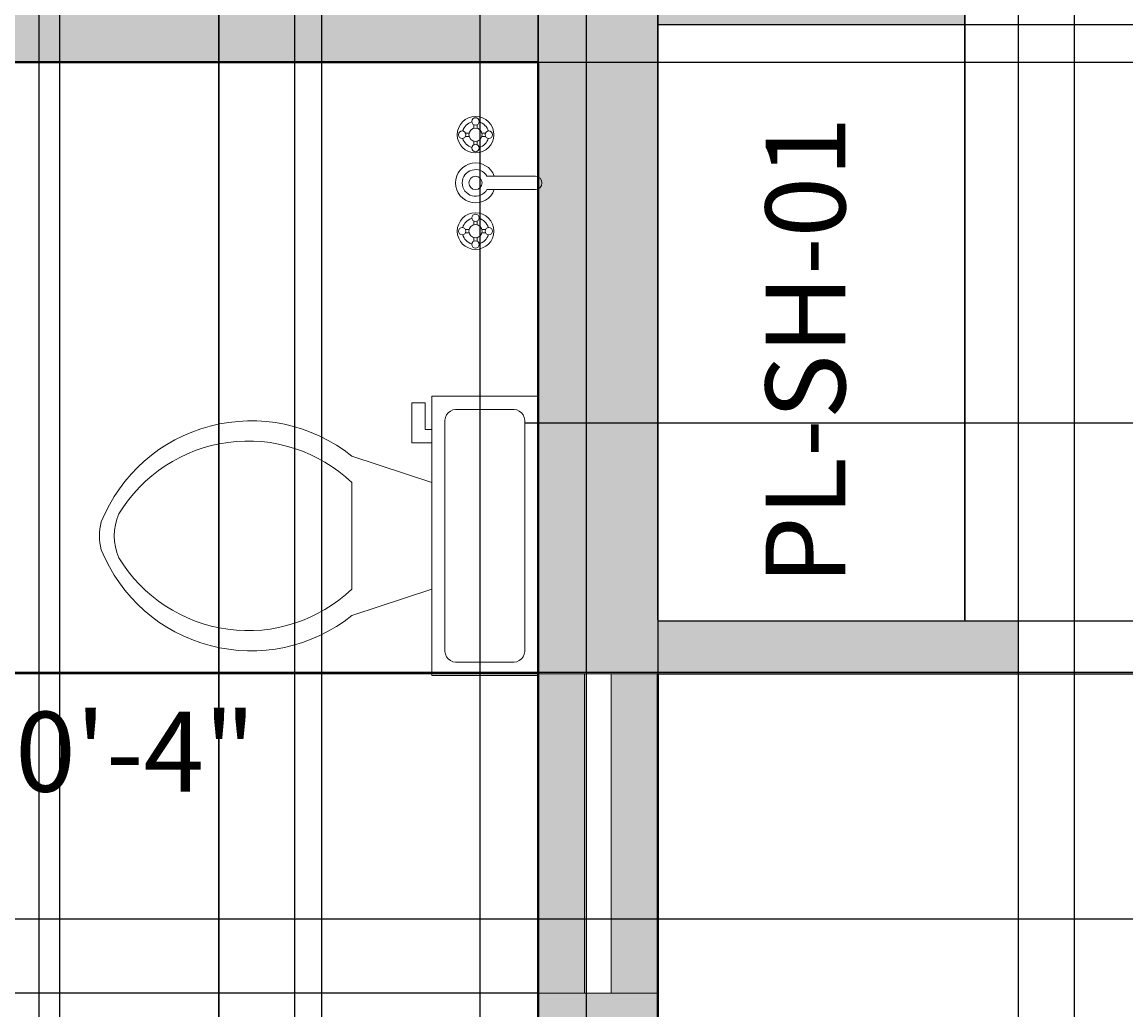
# Model space of a CAD drawing. Units: inches. Extents: x 818 to 1898, y 976 to 2364.
# Tile 46 of 96: x 1667 to 1750, y 1520 to 1594. Entities that reach past the tile are written whole.
import ezdxf

# ---------------------------------------------------------------- set-up
doc = ezdxf.new("R2010")
doc.units = ezdxf.units.IN
doc.header["$LTSCALE"] = 5
doc.header["$MEASUREMENT"] = 0
for name, color, linetype, lineweight in [('A-ANNO-DIMS', 2, 'Continuous', 18), ('A-ANNO-TEXT', 7, 'Continuous', 18), ('A-AREA-IDEN', 7, 'Continuous', 18), ('A-FLOR-FIXT', 9, 'Continuous', 18), ('A-FLOR-SHFT', 7, 'Continuous', 25), ('A-GLAZ', 4, 'Continuous', 18), ('A-WALL', 7, 'Continuous', 40)]:
    doc.layers.add(name, color=color, linetype=linetype, lineweight=lineweight)
doc.layers.add('A-GLAZ-PATT', color=141, linetype='Continuous', lineweight=9, true_color=0xadddf7)
doc.layers.add('A-WALL-PATT', color=251, linetype='Continuous', lineweight=13, true_color=0x636466)
doc.styles.get("Standard").update_dxf_attribs({"font": 'arial.ttf'})
doc.dimstyles.get("Standard").update_dxf_attribs({"dimtxt": 0.18, "dimasz": 0.18, "dimexe": 0.18, "dimexo": 0.0625, "dimgap": 0.09, "dimtad": 0, "dimtih": 1, "dimtoh": 1, "dimdec": 4, "dimzin": 0, "dimdsep": 46, "dimtxsty": 'Standard', "dimcen": 0.09, "dimadec": 0, "dimazin": 0, "dimtfac": 1, "dimtdec": 4, "dimtofl": 0, "dimtmove": 0, "dimatfit": 3, "dimfxl": 1, "dimtolj": 1, "dimtzin": 0, "dimarcsym": 0})

# ---------------------------------------------------------------- blocks, each defined once
blk = doc.blocks.new('Toilet - top')
for p, q in [((9.5, -6), (9.5, -2)), ((-8, -8.5), (-8, -8)), ((-7, -8), (-7, -9.5)), ((-4, -8), (-6, -14)), ((4, -8), (6, -14)), ((-10, -8.5), (-8, -8.5)), ((-10, -9.5), (-10, -8.5)), ((-7, -9.5), (-10, -9.5)), ((4, -14), (-4, -14))]:
    blk.add_line(p, q)
blk.add_lwpolyline([(10.5, -8), (10.5, 0), (-10.5, 0), (-10.5, -8)], close=True)
for points in [[(8.5, -1), (-8.5, -1)], [(-9.5, -2), (-9.5, -6)], [(-8.5, -7), (8.5, -7)]]:
    blk.add_lwpolyline(points)
for centre, radius, start, end in [((-8.625, -1.875), 0.884, 81.8699, 188.1301), ((8.625, -1.875), 0.884, 351.8699, 98.1301), ((-8.625, -6.125), 0.884, 171.8699, 278.1301), ((8.625, -6.125), 0.884, 261.8699, 8.1301), ((3.52, -21.58), 12.169, 141.46911, 247.97143), ((4.2, -21.817), 11.329, 136.36773, 238.94682), ((-3.519, -21.58), 12.169, 292.02843, 38.53071), ((-4.2, -21.817), 11.329, 301.05301, 43.63209), ((0, -27.876), 4, 245.73182, 294.26817), ((0, -29), 4, 254.86053, 285.13947)]:
    blk.add_arc(centre, radius, start, end)
blk = doc.blocks.new('Faucet - Bathroom top')
for p, q in [((-4.107, 0.125), (-4.375, 0.125)), ((-3.75, 0.4788), (-3.75, 0.75)), ((-3.5, 0.482), (-3.5, 0.75)), ((-3.1461, 0.125), (-2.875, 0.125)), ((3.143, 0.125), (2.875, 0.125)), ((3.5, 0.4788), (3.5, 0.75)), ((3.75, 0.482), (3.75, 0.75)), ((4.1039, 0.125), (4.375, 0.125)), ((-4.1039, -0.125), (-4.375, -0.125)), ((-3.75, -0.4821), (-3.75, -0.75)), ((-3.5, -0.4789), (-3.5, -0.75)), ((-3.143, -0.125), (-2.875, -0.125)), ((3.1461, -0.125), (2.875, -0.125)), ((3.5, -0.4821), (3.5, -0.75)), ((3.75, -0.4789), (3.75, -0.75)), ((4.107, -0.125), (4.375, -0.125)), ((-0.5, -0.8639), (-0.5, -4.5)), ((0.5, -4.5), (0.5, -0.8631))]:
    blk.add_line(p, q)
for centre, radius in [((-3.625, 0), 1.375), ((-3.625, 1), 0.2795), ((3.625, 0), 1.375), ((3.625, 1), 0.2795), ((-4.625, 0), 0.2795), ((-3.625, 0), 0.5), ((-2.625, 0), 0.2795), ((0, 0), 0.5), ((2.625, 0), 0.2795), ((3.625, 0), 0.5), ((4.625, 0), 0.2795), ((-3.625, -1), 0.2795), ((3.625, -1), 0.2795)]:
    blk.add_circle(centre, radius)
for centre, radius, start, end in [((-3.625, 0), 1, 105.2407, 164.2093), ((-3.625, 0), 1, 16.44125, 74.07887), ((0, 0), 1.5, 289.6514, 250.3603), ((0, 0), 1, 300.3431, 239.7554), ((3.625, 0), 1, 106.12, 164.0884), ((3.625, 0), 1, 16.23422, 73.90469), ((-3.625, 0), 1, 196.2342, 253.9047), ((-3.625, 0), 1, 286.12, 344.0884), ((3.625, 0), 1, 196.4413, 254.0789), ((3.625, 0), 1, 285.2407, 344.2093), ((0, -4.5), 0.5, 180, 0)]:
    blk.add_arc(centre, radius, start, end)
blk = doc.blocks.new('*D71')
at = {"layer": 'A-ANNO-DIMS', "color": 0, "lineweight": -2, "ltscale": 5, "transparency": 16777216}
for p, q in [((1714.788, 2053.078), (1897.916, 2053.078)), ((1897.736, 2052.898), (1897.736, 1699.76)), ((1897.736, 1346.258), (1897.736, 1699.396)), ((1714.788, 1346.078), (1897.916, 1346.078))]:
    blk.add_line(p, q, dxfattribs=at)
at = {"layer": 'A-ANNO-DIMS', "color": 0, "ltscale": 5, "transparency": 16777216}
for points in [[(1897.706, 2052.898), (1897.766, 2052.898), (1897.736, 2053.078)], [(1897.706, 1346.258), (1897.766, 1346.258), (1897.736, 1346.078)]]:
    blk.add_solid(points, dxfattribs=at)
at = {"layer": 'Defpoints', "color": 0, "ltscale": 5, "transparency": 16777216}
for p in [(1714.725, 2053.078), (1897.736, 2053.078), (1714.725, 1346.078)]:
    blk.add_point(p, dxfattribs=at)
at = {"layer": 'A-ANNO-DIMS', "color": 0, "ltscale": 5, "transparency": 16777216, "insert": (1897.736, 1699.578), "char_height": 0.18, "attachment_point": 5}
blk.add_mtext('\\A1;707', dxfattribs=at)
blk = doc.blocks.new('*D103')
at = {"layer": 'A-ANNO-DIMS', "color": 0, "lineweight": -2, "ltscale": 5, "transparency": 16777216}
for p, q in [((1626.575, 1071.118), (1626.575, 2363.873)), ((1626.755, 2363.693), (1657.699, 2363.693)), ((1689.291, 2363.693), (1658.348, 2363.693)), ((1689.471, 1071.118), (1689.471, 2363.873))]:
    blk.add_line(p, q, dxfattribs=at)
at = {"layer": 'A-ANNO-DIMS', "color": 0, "ltscale": 5, "transparency": 16777216}
for points in [[(1626.755, 2363.723), (1626.755, 2363.663), (1626.575, 2363.693)], [(1689.291, 2363.723), (1689.291, 2363.663), (1689.471, 2363.693)]]:
    blk.add_solid(points, dxfattribs=at)
at = {"layer": 'Defpoints', "color": 0, "ltscale": 5, "transparency": 16777216}
for p in [(1689.471, 2363.693), (1626.575, 1071.055), (1689.471, 1071.055)]:
    blk.add_point(p, dxfattribs=at)
at = {"layer": 'A-ANNO-DIMS', "color": 0, "ltscale": 5, "transparency": 16777216, "insert": (1658.023, 2363.693), "char_height": 0.18, "attachment_point": 5}
blk.add_mtext('\\A1;62.9', dxfattribs=at)
blk = doc.blocks.new('*D104')
at = {"layer": 'A-ANNO-DIMS', "color": 0, "lineweight": -2, "ltscale": 5, "transparency": 16777216}
for p, q in [((1689.471, 1071.118), (1689.471, 2363.873)), ((1689.651, 2363.693), (1717.401, 2363.693)), ((1745.903, 2363.693), (1718.154, 2363.693)), ((1746.083, 1071.118), (1746.083, 2363.873))]:
    blk.add_line(p, q, dxfattribs=at)
at = {"layer": 'A-ANNO-DIMS', "color": 0, "ltscale": 5, "transparency": 16777216}
for points in [[(1689.651, 2363.723), (1689.651, 2363.663), (1689.471, 2363.693)], [(1745.903, 2363.723), (1745.903, 2363.663), (1746.083, 2363.693)]]:
    blk.add_solid(points, dxfattribs=at)
at = {"layer": 'Defpoints', "color": 0, "ltscale": 5, "transparency": 16777216}
for p in [(1746.083, 2363.693), (1689.471, 1071.055), (1746.083, 1071.055)]:
    blk.add_point(p, dxfattribs=at)
at = {"layer": 'A-ANNO-DIMS', "color": 0, "ltscale": 5, "transparency": 16777216, "insert": (1717.777, 2363.693), "char_height": 0.18, "attachment_point": 5}
blk.add_mtext('\\A1;56.61', dxfattribs=at)
blk = doc.blocks.new('*D117')
at = {"layer": 'A-ANNO-DIMS', "color": 0, "lineweight": -2, "ltscale": 5, "transparency": 16777216}
for p, q in [((1766.29, 1545.183), (818.026, 1545.183)), ((818.206, 1545.003), (818.206, 1501.178)), ((818.206, 1456.989), (818.206, 1500.814)), ((1766.29, 1456.809), (818.026, 1456.809))]:
    blk.add_line(p, q, dxfattribs=at)
at = {"layer": 'A-ANNO-DIMS', "color": 0, "ltscale": 5, "transparency": 16777216}
for points in [[(818.176, 1545.003), (818.236, 1545.003), (818.206, 1545.183)], [(818.176, 1456.989), (818.236, 1456.989), (818.206, 1456.809)]]:
    blk.add_solid(points, dxfattribs=at)
at = {"layer": 'Defpoints', "color": 0, "ltscale": 5, "transparency": 16777216}
for p in [(818.206, 1545.183), (1766.352, 1545.183), (1766.352, 1456.809)]:
    blk.add_point(p, dxfattribs=at)
at = {"layer": 'A-ANNO-DIMS', "color": 0, "ltscale": 5, "transparency": 16777216, "insert": (818.206, 1500.996), "char_height": 0.18, "attachment_point": 5}
blk.add_mtext('\\A1;88.37', dxfattribs=at)
blk = doc.blocks.new('*D118')
at = {"layer": 'A-ANNO-DIMS', "color": 0, "lineweight": -2, "ltscale": 5, "transparency": 16777216}
for p, q in [((1766.29, 1627.505), (818.026, 1627.505)), ((818.206, 1627.325), (818.206, 1586.526)), ((818.206, 1545.363), (818.206, 1586.162)), ((1766.29, 1545.183), (818.026, 1545.183))]:
    blk.add_line(p, q, dxfattribs=at)
at = {"layer": 'A-ANNO-DIMS', "color": 0, "ltscale": 5, "transparency": 16777216}
for points in [[(818.176, 1627.325), (818.236, 1627.325), (818.206, 1627.505)], [(818.176, 1545.363), (818.236, 1545.363), (818.206, 1545.183)]]:
    blk.add_solid(points, dxfattribs=at)
at = {"layer": 'Defpoints', "color": 0, "ltscale": 5, "transparency": 16777216}
for p in [(818.206, 1627.505), (1766.352, 1627.505), (1766.352, 1545.183)]:
    blk.add_point(p, dxfattribs=at)
at = {"layer": 'A-ANNO-DIMS', "color": 0, "ltscale": 5, "transparency": 16777216, "insert": (818.206, 1586.344), "char_height": 0.18, "attachment_point": 5}
blk.add_mtext('\\A1;82.32', dxfattribs=at)
blk = doc.blocks.new('*D154')
at = {"layer": 'A-ANNO-DIMS', "color": 0, "lineweight": -2, "ltscale": 5, "transparency": 16777216}
for p, q in [((1701.369, 1290.141), (1701.369, 2363.873)), ((1701.549, 2363.693), (1705.22, 2363.693)), ((1709.189, 2363.693), (1705.518, 2363.693)), ((1709.369, 1298.141), (1709.369, 2363.873))]:
    blk.add_line(p, q, dxfattribs=at)
at = {"layer": 'A-ANNO-DIMS', "color": 0, "ltscale": 5, "transparency": 16777216}
for points in [[(1701.549, 2363.723), (1701.549, 2363.663), (1701.369, 2363.693)], [(1709.189, 2363.723), (1709.189, 2363.663), (1709.369, 2363.693)]]:
    blk.add_solid(points, dxfattribs=at)
at = {"layer": 'Defpoints', "color": 0, "ltscale": 5, "transparency": 16777216}
for p in [(1709.369, 2363.693), (1709.369, 1298.078), (1701.369, 1290.078)]:
    blk.add_point(p, dxfattribs=at)
at = {"layer": 'A-ANNO-DIMS', "color": 0, "ltscale": 5, "transparency": 16777216, "insert": (1705.369, 2363.693), "char_height": 0.18, "attachment_point": 5}
blk.add_mtext('\\A1;8', dxfattribs=at)
blk = doc.blocks.new('*D170')
at = {"layer": 'A-ANNO-DIMS', "color": 0, "lineweight": -2, "ltscale": 5, "transparency": 16777216}
for p, q in [((1430.788, 1600.078), (1897.916, 1600.078)), ((1897.736, 1599.898), (1897.736, 1550.76)), ((1897.736, 1501.258), (1897.736, 1550.396)), ((1430.788, 1501.078), (1897.916, 1501.078))]:
    blk.add_line(p, q, dxfattribs=at)
at = {"layer": 'A-ANNO-DIMS', "color": 0, "ltscale": 5, "transparency": 16777216}
for points in [[(1897.706, 1599.898), (1897.766, 1599.898), (1897.736, 1600.078)], [(1897.706, 1501.258), (1897.766, 1501.258), (1897.736, 1501.078)]]:
    blk.add_solid(points, dxfattribs=at)
at = {"layer": 'Defpoints', "color": 0, "ltscale": 5, "transparency": 16777216}
for p in [(1430.725, 1600.078), (1897.736, 1600.078), (1430.725, 1501.078)]:
    blk.add_point(p, dxfattribs=at)
at = {"layer": 'A-ANNO-DIMS', "color": 0, "ltscale": 5, "transparency": 16777216, "insert": (1897.736, 1550.578), "char_height": 0.18, "attachment_point": 5}
blk.add_mtext('\\A1;99', dxfattribs=at)
blk = doc.blocks.new('*D178')
at = {"layer": 'A-ANNO-DIMS', "color": 0, "lineweight": -2, "ltscale": 5, "transparency": 16777216}
for p, q in [((1669.725, 1600.016), (1669.725, 975.663)), ((1705.725, 1600.016), (1705.725, 975.663)), ((1669.905, 975.843), (1687.506, 975.843)), ((1705.545, 975.843), (1687.944, 975.843))]:
    blk.add_line(p, q, dxfattribs=at)
at = {"layer": 'A-ANNO-DIMS', "color": 0, "ltscale": 5, "transparency": 16777216}
for points in [[(1669.905, 975.873), (1669.905, 975.813), (1669.725, 975.843)], [(1705.545, 975.873), (1705.545, 975.813), (1705.725, 975.843)]]:
    blk.add_solid(points, dxfattribs=at)
at = {"layer": 'Defpoints', "color": 0, "ltscale": 5, "transparency": 16777216}
for p in [(1669.725, 1600.078), (1705.725, 1600.078), (1705.725, 975.843)]:
    blk.add_point(p, dxfattribs=at)
at = {"layer": 'A-ANNO-DIMS', "color": 0, "ltscale": 5, "transparency": 16777216, "insert": (1687.725, 975.843), "char_height": 0.18, "attachment_point": 5}
blk.add_mtext('\\A1;36', dxfattribs=at)
blk = doc.blocks.new('*D180')
at = {"layer": 'A-ANNO-DIMS', "color": 0, "lineweight": -2, "ltscale": 5, "transparency": 16777216}
for p, q in [((1599.725, 1639.516), (1599.725, 975.663)), ((1669.725, 1639.516), (1669.725, 975.663)), ((1599.905, 975.843), (1634.507, 975.843)), ((1669.545, 975.843), (1634.943, 975.843))]:
    blk.add_line(p, q, dxfattribs=at)
at = {"layer": 'A-ANNO-DIMS', "color": 0, "ltscale": 5, "transparency": 16777216}
for points in [[(1599.905, 975.873), (1599.905, 975.813), (1599.725, 975.843)], [(1669.545, 975.873), (1669.545, 975.813), (1669.725, 975.843)]]:
    blk.add_solid(points, dxfattribs=at)
at = {"layer": 'Defpoints', "color": 0, "ltscale": 5, "transparency": 16777216}
for p in [(1599.725, 1639.578), (1669.725, 1639.578), (1669.725, 975.843)]:
    blk.add_point(p, dxfattribs=at)
at = {"layer": 'A-ANNO-DIMS', "color": 0, "ltscale": 5, "transparency": 16777216, "insert": (1634.725, 975.843), "char_height": 0.18, "attachment_point": 5}
blk.add_mtext('\\A1;70', dxfattribs=at)
blk = doc.blocks.new('*D183')
at = {"layer": 'A-ANNO-DIMS', "color": 0, "lineweight": -2, "ltscale": 5, "transparency": 16777216}
for p, q in [((1714.725, 1545.016), (1714.725, 975.663)), ((1741.841, 1545.016), (1741.841, 975.663)), ((1714.905, 975.843), (1727.818, 975.843)), ((1741.661, 975.843), (1728.748, 975.843))]:
    blk.add_line(p, q, dxfattribs=at)
at = {"layer": 'A-ANNO-DIMS', "color": 0, "ltscale": 5, "transparency": 16777216}
for points in [[(1714.905, 975.873), (1714.905, 975.813), (1714.725, 975.843)], [(1741.661, 975.873), (1741.661, 975.813), (1741.841, 975.843)]]:
    blk.add_solid(points, dxfattribs=at)
at = {"layer": 'Defpoints', "color": 0, "ltscale": 5, "transparency": 16777216}
for p in [(1714.725, 1545.078), (1741.841, 1545.078), (1741.841, 975.843)]:
    blk.add_point(p, dxfattribs=at)
at = {"layer": 'A-ANNO-DIMS', "color": 0, "ltscale": 5, "transparency": 16777216, "insert": (1728.283, 975.843), "char_height": 0.18, "attachment_point": 5}
blk.add_mtext('\\A1;27.116', dxfattribs=at)
blk = doc.blocks.new('*D184')
at = {"layer": 'A-ANNO-DIMS', "color": 0, "lineweight": -2, "ltscale": 5, "transparency": 16777216}
for p, q in [((1737.903, 1593.918), (1897.916, 1593.918)), ((1897.736, 1593.738), (1897.736, 1571.68)), ((1897.736, 1549.258), (1897.736, 1571.316)), ((1737.903, 1549.078), (1897.916, 1549.078))]:
    blk.add_line(p, q, dxfattribs=at)
at = {"layer": 'A-ANNO-DIMS', "color": 0, "ltscale": 5, "transparency": 16777216}
for points in [[(1897.706, 1593.738), (1897.766, 1593.738), (1897.736, 1593.918)], [(1897.706, 1549.258), (1897.766, 1549.258), (1897.736, 1549.078)]]:
    blk.add_solid(points, dxfattribs=at)
at = {"layer": 'Defpoints', "color": 0, "ltscale": 5, "transparency": 16777216}
for p in [(1737.841, 1593.918), (1897.736, 1593.918), (1737.841, 1549.078)]:
    blk.add_point(p, dxfattribs=at)
at = {"layer": 'A-ANNO-DIMS', "color": 0, "ltscale": 5, "transparency": 16777216, "insert": (1897.736, 1571.498), "char_height": 0.18, "attachment_point": 5}
blk.add_mtext('\\A1;44.84', dxfattribs=at)
blk = doc.blocks.new('*D186')
at = {"layer": 'A-ANNO-DIMS', "color": 0, "lineweight": -2, "ltscale": 5, "transparency": 16777216}
for p, q in [((1714.725, 1549.141), (1714.725, 2363.873)), ((1714.905, 2363.693), (1725.818, 2363.693)), ((1737.661, 2363.693), (1726.748, 2363.693)), ((1737.841, 1549.141), (1737.841, 2363.873))]:
    blk.add_line(p, q, dxfattribs=at)
at = {"layer": 'A-ANNO-DIMS', "color": 0, "ltscale": 5, "transparency": 16777216}
for points in [[(1714.905, 2363.723), (1714.905, 2363.663), (1714.725, 2363.693)], [(1737.661, 2363.723), (1737.661, 2363.663), (1737.841, 2363.693)]]:
    blk.add_solid(points, dxfattribs=at)
at = {"layer": 'Defpoints', "color": 0, "ltscale": 5, "transparency": 16777216}
for p in [(1737.841, 2363.693), (1714.725, 1549.078), (1737.841, 1549.078)]:
    blk.add_point(p, dxfattribs=at)
at = {"layer": 'A-ANNO-DIMS', "color": 0, "ltscale": 5, "transparency": 16777216, "insert": (1726.283, 2363.693), "char_height": 0.18, "attachment_point": 5}
blk.add_mtext('\\A1;23.116', dxfattribs=at)
blk = doc.blocks.new('*D187')
at = {"layer": 'A-ANNO-DIMS', "color": 0, "lineweight": -2, "ltscale": 5, "transparency": 16777216}
for p, q in [((1705.663, 1545.078), (818.026, 1545.078)), ((818.206, 1544.898), (818.206, 1533.259)), ((818.206, 1521.258), (818.206, 1532.898)), ((1705.663, 1521.078), (818.026, 1521.078))]:
    blk.add_line(p, q, dxfattribs=at)
at = {"layer": 'A-ANNO-DIMS', "color": 0, "ltscale": 5, "transparency": 16777216}
for points in [[(818.176, 1544.898), (818.236, 1544.898), (818.206, 1545.078)], [(818.176, 1521.258), (818.236, 1521.258), (818.206, 1521.078)]]:
    blk.add_solid(points, dxfattribs=at)
at = {"layer": 'Defpoints', "color": 0, "ltscale": 5, "transparency": 16777216}
for p in [(818.206, 1545.078), (1705.725, 1545.078), (1705.725, 1521.078)]:
    blk.add_point(p, dxfattribs=at)
at = {"layer": 'A-ANNO-DIMS', "color": 0, "ltscale": 5, "transparency": 16777216, "insert": (818.206, 1533.078), "char_height": 0.18, "attachment_point": 5}
blk.add_mtext('\\A1;24', dxfattribs=at)
blk = doc.blocks.new('*D188')
at = {"layer": 'A-ANNO-DIMS', "color": 0, "lineweight": -2, "ltscale": 5, "transparency": 16777216}
for p, q in [((1714.788, 1545.078), (1897.916, 1545.078)), ((1897.736, 1544.898), (1897.736, 1445.76)), ((1897.736, 1346.258), (1897.736, 1445.396)), ((1714.788, 1346.078), (1897.916, 1346.078))]:
    blk.add_line(p, q, dxfattribs=at)
at = {"layer": 'A-ANNO-DIMS', "color": 0, "ltscale": 5, "transparency": 16777216}
for points in [[(1897.706, 1544.898), (1897.766, 1544.898), (1897.736, 1545.078)], [(1897.706, 1346.258), (1897.766, 1346.258), (1897.736, 1346.078)]]:
    blk.add_solid(points, dxfattribs=at)
at = {"layer": 'Defpoints', "color": 0, "ltscale": 5, "transparency": 16777216}
for p in [(1714.725, 1545.078), (1897.736, 1545.078), (1714.725, 1346.078)]:
    blk.add_point(p, dxfattribs=at)
at = {"layer": 'A-ANNO-DIMS', "color": 0, "ltscale": 5, "transparency": 16777216, "insert": (1897.736, 1445.578), "char_height": 0.18, "attachment_point": 5}
blk.add_mtext('\\A1;199', dxfattribs=at)
blk = doc.blocks.new('*D195')
at = {"layer": 'A-ANNO-DIMS', "color": 0, "lineweight": -2, "ltscale": 5, "transparency": 16777216}
for p, q in [((1681.725, 1379.141), (1681.725, 2363.873)), ((1681.905, 2363.693), (1693.505, 2363.693)), ((1705.545, 2363.693), (1693.945, 2363.693)), ((1705.725, 1355.141), (1705.725, 2363.873))]:
    blk.add_line(p, q, dxfattribs=at)
at = {"layer": 'A-ANNO-DIMS', "color": 0, "ltscale": 5, "transparency": 16777216}
for points in [[(1681.905, 2363.723), (1681.905, 2363.663), (1681.725, 2363.693)], [(1705.545, 2363.723), (1705.545, 2363.663), (1705.725, 2363.693)]]:
    blk.add_solid(points, dxfattribs=at)
at = {"layer": 'Defpoints', "color": 0, "ltscale": 5, "transparency": 16777216}
for p in [(1705.725, 2363.693), (1681.725, 1379.078), (1705.725, 1355.078)]:
    blk.add_point(p, dxfattribs=at)
at = {"layer": 'A-ANNO-DIMS', "color": 0, "ltscale": 5, "transparency": 16777216, "insert": (1693.725, 2363.693), "char_height": 0.18, "attachment_point": 5}
blk.add_mtext('\\A1;24', dxfattribs=at)
blk = doc.blocks.new('*D197')
at = {"layer": 'A-ANNO-DIMS', "color": 0, "lineweight": -2, "ltscale": 5, "transparency": 16777216}
for p, q in [((1457.788, 1526.671), (1897.916, 1526.671)), ((1897.736, 1526.491), (1897.736, 1468.076)), ((1897.736, 1409.298), (1897.736, 1467.713)), ((1457.788, 1409.118), (1897.916, 1409.118))]:
    blk.add_line(p, q, dxfattribs=at)
at = {"layer": 'A-ANNO-DIMS', "color": 0, "ltscale": 5, "transparency": 16777216}
for points in [[(1897.706, 1526.491), (1897.766, 1526.491), (1897.736, 1526.671)], [(1897.706, 1409.298), (1897.766, 1409.298), (1897.736, 1409.118)]]:
    blk.add_solid(points, dxfattribs=at)
at = {"layer": 'Defpoints', "color": 0, "ltscale": 5, "transparency": 16777216}
for p in [(1457.725, 1526.671), (1897.736, 1526.671), (1457.725, 1409.118)]:
    blk.add_point(p, dxfattribs=at)
at = {"layer": 'A-ANNO-DIMS', "color": 0, "ltscale": 5, "transparency": 16777216, "insert": (1897.736, 1467.894), "char_height": 0.18, "attachment_point": 5}
blk.add_mtext('\\A1;117.55', dxfattribs=at)
blk = doc.blocks.new('*D198')
at = {"layer": 'A-ANNO-DIMS', "color": 0, "lineweight": -2, "ltscale": 5, "transparency": 16777216}
for p, q in [((1741.841, 1545.016), (1741.841, 975.663)), ((1430.725, 1346.016), (1430.725, 975.663)), ((1430.905, 975.843), (1585.907, 975.843)), ((1741.661, 975.843), (1586.659, 975.843))]:
    blk.add_line(p, q, dxfattribs=at)
at = {"layer": 'A-ANNO-DIMS', "color": 0, "ltscale": 5, "transparency": 16777216}
for points in [[(1430.905, 975.873), (1430.905, 975.813), (1430.725, 975.843)], [(1741.661, 975.873), (1741.661, 975.813), (1741.841, 975.843)]]:
    blk.add_solid(points, dxfattribs=at)
at = {"layer": 'Defpoints', "color": 0, "ltscale": 5, "transparency": 16777216}
for p in [(1741.841, 1545.078), (1430.725, 1346.078), (1741.841, 975.843)]:
    blk.add_point(p, dxfattribs=at)
at = {"layer": 'A-ANNO-DIMS', "color": 0, "ltscale": 5, "transparency": 16777216, "insert": (1586.283, 975.843), "char_height": 0.18, "attachment_point": 5}
blk.add_mtext('\\A1;311.1', dxfattribs=at)
blk = doc.blocks.new('*D199')
at = {"layer": 'A-ANNO-DIMS', "color": 0, "lineweight": -2, "ltscale": 5, "transparency": 16777216}
for p, q in [((1559.788, 1687.078), (1897.916, 1687.078)), ((1897.736, 1686.898), (1897.736, 1513.154)), ((1897.736, 1339.045), (1897.736, 1512.79)), ((1660.377, 1338.865), (1897.916, 1338.865))]:
    blk.add_line(p, q, dxfattribs=at)
at = {"layer": 'A-ANNO-DIMS', "color": 0, "ltscale": 5, "transparency": 16777216}
for points in [[(1897.706, 1686.898), (1897.766, 1686.898), (1897.736, 1687.078)], [(1897.706, 1339.045), (1897.766, 1339.045), (1897.736, 1338.865)]]:
    blk.add_solid(points, dxfattribs=at)
at = {"layer": 'Defpoints', "color": 0, "ltscale": 5, "transparency": 16777216}
for p in [(1559.725, 1687.078), (1897.736, 1687.078), (1660.314, 1338.865)]:
    blk.add_point(p, dxfattribs=at)
at = {"layer": 'A-ANNO-DIMS', "color": 0, "ltscale": 5, "transparency": 16777216, "insert": (1897.736, 1512.972), "char_height": 0.18, "attachment_point": 5}
blk.add_mtext('\\A1;348.2', dxfattribs=at)
blk = doc.blocks.new('*D202')
at = {"layer": 'A-ANNO-DIMS', "color": 0, "lineweight": -2, "ltscale": 5, "transparency": 16777216}
for p, q in [((1705.788, 1591.078), (1897.916, 1591.078)), ((1897.736, 1590.898), (1897.736, 1577.702)), ((1897.736, 1564.146), (1897.736, 1577.342)), ((1704.788, 1563.966), (1897.916, 1563.966))]:
    blk.add_line(p, q, dxfattribs=at)
at = {"layer": 'A-ANNO-DIMS', "color": 0, "ltscale": 5, "transparency": 16777216}
for points in [[(1897.706, 1590.898), (1897.766, 1590.898), (1897.736, 1591.078)], [(1897.706, 1564.146), (1897.766, 1564.146), (1897.736, 1563.966)]]:
    blk.add_solid(points, dxfattribs=at)
at = {"layer": 'Defpoints', "color": 0, "ltscale": 5, "transparency": 16777216}
for p in [(1705.725, 1591.078), (1897.736, 1591.078), (1704.725, 1563.966)]:
    blk.add_point(p, dxfattribs=at)
at = {"layer": 'A-ANNO-DIMS', "color": 0, "ltscale": 5, "transparency": 16777216, "insert": (1897.736, 1577.522), "char_height": 0.18, "attachment_point": 5}
blk.add_mtext('\\A1;27.11', dxfattribs=at)
blk = doc.blocks.new('*D212')
at = {"layer": 'A-ANNO-DIMS', "color": 0, "lineweight": -2, "ltscale": 5, "transparency": 16777216}
for p, q in [((1681.725, 1900.016), (1681.725, 975.663)), ((1705.725, 1876.016), (1705.725, 975.663)), ((1681.905, 975.843), (1693.505, 975.843)), ((1705.545, 975.843), (1693.945, 975.843))]:
    blk.add_line(p, q, dxfattribs=at)
at = {"layer": 'A-ANNO-DIMS', "color": 0, "ltscale": 5, "transparency": 16777216}
for points in [[(1681.905, 975.873), (1681.905, 975.813), (1681.725, 975.843)], [(1705.545, 975.873), (1705.545, 975.813), (1705.725, 975.843)]]:
    blk.add_solid(points, dxfattribs=at)
at = {"layer": 'Defpoints', "color": 0, "ltscale": 5, "transparency": 16777216}
for p in [(1681.725, 1900.078), (1705.725, 1876.078), (1705.725, 975.843)]:
    blk.add_point(p, dxfattribs=at)
at = {"layer": 'A-ANNO-DIMS', "color": 0, "ltscale": 5, "transparency": 16777216, "insert": (1693.725, 975.843), "char_height": 0.18, "attachment_point": 5}
blk.add_mtext('\\A1;24', dxfattribs=at)
blk = doc.blocks.new('*D214')
at = {"layer": 'A-ANNO-DIMS', "color": 0, "lineweight": -2, "ltscale": 5, "transparency": 16777216}
for p, q in [((1511.725, 1687.016), (1511.725, 975.663)), ((1714.725, 1687.016), (1714.725, 975.663)), ((1511.905, 975.843), (1612.935, 975.843)), ((1714.545, 975.843), (1613.516, 975.843))]:
    blk.add_line(p, q, dxfattribs=at)
at = {"layer": 'A-ANNO-DIMS', "color": 0, "ltscale": 5, "transparency": 16777216}
for points in [[(1511.905, 975.873), (1511.905, 975.813), (1511.725, 975.843)], [(1714.545, 975.873), (1714.545, 975.813), (1714.725, 975.843)]]:
    blk.add_solid(points, dxfattribs=at)
at = {"layer": 'Defpoints', "color": 0, "ltscale": 5, "transparency": 16777216}
for p in [(1511.725, 1687.078), (1714.725, 1687.078), (1714.725, 975.843)]:
    blk.add_point(p, dxfattribs=at)
at = {"layer": 'A-ANNO-DIMS', "color": 0, "ltscale": 5, "transparency": 16777216, "insert": (1613.225, 975.843), "char_height": 0.18, "attachment_point": 5}
blk.add_mtext('\\A1;203', dxfattribs=at)
blk = doc.blocks.new('*D221')
at = {"layer": 'A-ANNO-DIMS', "color": 0, "lineweight": -2, "ltscale": 5, "transparency": 16777216}
for p, q in [((1668.184, 1696.016), (1668.184, 975.663)), ((1705.725, 1696.016), (1705.725, 975.663)), ((1668.364, 975.843), (1686.561, 975.843)), ((1705.545, 975.843), (1687.348, 975.843))]:
    blk.add_line(p, q, dxfattribs=at)
at = {"layer": 'A-ANNO-DIMS', "color": 0, "ltscale": 5, "transparency": 16777216}
for points in [[(1668.364, 975.873), (1668.364, 975.813), (1668.184, 975.843)], [(1705.545, 975.873), (1705.545, 975.813), (1705.725, 975.843)]]:
    blk.add_solid(points, dxfattribs=at)
at = {"layer": 'Defpoints', "color": 0, "ltscale": 5, "transparency": 16777216}
for p in [(1668.184, 1696.078), (1705.725, 1696.078), (1705.725, 975.843)]:
    blk.add_point(p, dxfattribs=at)
at = {"layer": 'A-ANNO-DIMS', "color": 0, "ltscale": 5, "transparency": 16777216, "insert": (1686.955, 975.843), "char_height": 0.18, "attachment_point": 5}
blk.add_mtext('\\A1;37.54', dxfattribs=at)
blk = doc.blocks.new('*D228')
at = {"layer": 'A-ANNO-DIMS', "color": 0, "lineweight": -2, "ltscale": 5, "transparency": 16777216}
for p, q in [((1687.394, 1802.016), (1687.394, 975.663)), ((1705.725, 1802.016), (1705.725, 975.663)), ((1687.574, 975.843), (1696.174, 975.843)), ((1705.545, 975.843), (1696.945, 975.843))]:
    blk.add_line(p, q, dxfattribs=at)
at = {"layer": 'A-ANNO-DIMS', "color": 0, "ltscale": 5, "transparency": 16777216}
for points in [[(1687.574, 975.873), (1687.574, 975.813), (1687.394, 975.843)], [(1705.545, 975.873), (1705.545, 975.813), (1705.725, 975.843)]]:
    blk.add_solid(points, dxfattribs=at)
at = {"layer": 'Defpoints', "color": 0, "ltscale": 5, "transparency": 16777216}
for p in [(1687.394, 1802.078), (1705.725, 1802.078), (1705.725, 975.843)]:
    blk.add_point(p, dxfattribs=at)
at = {"layer": 'A-ANNO-DIMS', "color": 0, "ltscale": 5, "transparency": 16777216, "insert": (1696.56, 975.843), "char_height": 0.18, "attachment_point": 5}
blk.add_mtext('\\A1;18.33', dxfattribs=at)
blk = doc.blocks.new('*D267')
at = {"layer": 'A-ANNO-DIMS', "color": 0, "lineweight": -2, "ltscale": 5, "transparency": 16777216}
for p, q in [((1714.725, 1687.016), (1714.725, 975.663)), ((1741.841, 1687.016), (1741.841, 975.663)), ((1714.905, 975.843), (1727.818, 975.843)), ((1741.661, 975.843), (1728.748, 975.843))]:
    blk.add_line(p, q, dxfattribs=at)
at = {"layer": 'A-ANNO-DIMS', "color": 0, "ltscale": 5, "transparency": 16777216}
for points in [[(1714.905, 975.873), (1714.905, 975.813), (1714.725, 975.843)], [(1741.661, 975.873), (1741.661, 975.813), (1741.841, 975.843)]]:
    blk.add_solid(points, dxfattribs=at)
at = {"layer": 'Defpoints', "color": 0, "ltscale": 5, "transparency": 16777216}
for p in [(1714.725, 1687.078), (1741.841, 1687.078), (1741.841, 975.843)]:
    blk.add_point(p, dxfattribs=at)
at = {"layer": 'A-ANNO-DIMS', "color": 0, "ltscale": 5, "transparency": 16777216, "insert": (1728.283, 975.843), "char_height": 0.18, "attachment_point": 5}
blk.add_mtext('\\A1;27.116', dxfattribs=at)

msp = doc.modelspace()

# ---------------------------------------------------------------- hatches: boundary and pattern name
at = {"layer": 'A-GLAZ-PATT', "ltscale": 5}
h = msp.add_hatch(color=256, dxfattribs=at)
h.dxf.hatch_style = 1
h.paths.add_polyline_path([(1283.8183, 1504.5782), (1206.7252, 1504.5782), (1206.7252, 1501.0782), (1283.8183, 1501.0782)])
h.paths.add_polyline_path([(1283.8183, 1510.0782), (1206.7252, 1510.0782), (1206.7252, 1506.5782), (1283.8183, 1506.5782)])
h.paths.add_polyline_path([(1490.9163, 1355.0782), (1439.7252, 1355.0782), (1439.7252, 1409.0522), (1436.2252, 1409.0522), (1436.2252, 1351.5782), (1490.9163, 1351.5782)])
h.paths.add_polyline_path([(1434.2252, 1409.0522), (1430.7251, 1409.0522), (1430.7251, 1346.0782), (1435.0799, 1346.0782), (1435.0731, 1346.1152), (1435.1501, 1346.0782), (1490.9163, 1346.0782), (1490.9163, 1349.5782), (1434.2252, 1349.5782)])
h.paths.add_polyline_path([(1714.7251, 1545.0782), (1711.2252, 1545.0782), (1711.2252, 1521.0782), (1714.7251, 1521.0782)])
h.paths.add_polyline_path([(1709.2252, 1545.0782), (1705.7251, 1545.0782), (1705.7251, 1521.0782), (1709.2252, 1521.0782)])
h.paths.add_polyline_path([(1714.7251, 1687.0782), (1711.2252, 1687.0782), (1711.2252, 1649.9029), (1714.7251, 1649.9029)])
h.paths.add_polyline_path([(1709.2252, 1687.0782), (1705.7251, 1687.0782), (1705.7251, 1649.9029), (1709.2252, 1649.9029)])
h.paths.add_polyline_path([(1709.2252, 1745.5584), (1705.7251, 1745.5584), (1705.7251, 1717.3178), (1709.2252, 1717.3178)])
h.paths.add_polyline_path([(1714.7251, 1745.5584), (1711.2252, 1745.5584), (1711.2252, 1717.3178), (1714.7251, 1717.3178)])
h.paths.add_polyline_path([(1714.7251, 2014.5114), (1711.2252, 2014.5114), (1711.2252, 1962.0338), (1714.7251, 1962.0338)])
h.paths.add_polyline_path([(1709.2252, 2014.5114), (1705.7251, 2014.5114), (1705.7251, 1962.0338), (1709.2252, 1962.0338)])
h.paths.add_polyline_path([(1538.5155, 2047.5782), (1485.1216, 2047.5782), (1485.1216, 2044.0782), (1538.5155, 2044.0782)])
h.paths.add_polyline_path([(1538.5155, 2053.0782), (1485.1216, 2053.0782), (1485.1216, 2049.5782), (1538.5155, 2049.5782)])
h.paths.add_polyline_path([(1388.0315, 2047.5782), (1330.305, 2047.5782), (1330.305, 2044.0782), (1388.0315, 2044.0782)])
h.paths.add_polyline_path([(1388.0315, 2053.0782), (1330.305, 2053.0782), (1330.305, 2049.5782), (1388.0315, 2049.5782)])
h.paths.add_polyline_path([(1262.2252, 2019.2871), (1258.7252, 2019.2871), (1258.7252, 1928.9218), (1262.2252, 1928.9218)])
h.paths.add_polyline_path([(1267.7252, 2019.2871), (1264.2252, 2019.2871), (1264.2252, 1928.9218), (1267.7252, 1928.9218)])
h.paths.add_polyline_path([(1262.2252, 1862.9652), (1258.7252, 1862.9652), (1258.7252, 1814.9652), (1262.2252, 1814.9652)])
h.paths.add_polyline_path([(1267.7252, 1862.9652), (1264.2252, 1862.9652), (1264.2252, 1814.9652), (1267.7252, 1814.9652)])
h.paths.add_polyline_path([(1262.2252, 1755.3321), (1258.7252, 1755.3321), (1258.7252, 1707.3321), (1262.2252, 1707.3321)])
h.paths.add_polyline_path([(1267.7252, 1755.3321), (1264.2252, 1755.3321), (1264.2252, 1707.3321), (1267.7252, 1707.3321)])
h.paths.add_polyline_path([(1251.9333, 1692.5782), (1206.7252, 1692.5782), (1206.7252, 1687.0782), (1251.9333, 1687.0782)])
h.paths.add_polyline_path([(1251.9333, 1700.0782), (1206.7252, 1700.0782), (1206.7252, 1694.5782), (1251.9333, 1694.5782)])
at = {"layer": 'A-WALL-PATT', "ltscale": 5}
h = msp.add_hatch(color=256, dxfattribs=at)
h.dxf.hatch_style = 1
h.paths.add_polyline_path([(1267.7252, 1928.9218), (1258.7252, 1928.9218), (1258.7252, 1913.6401), (1250.3029, 1913.6401), (1250.3029, 1878.3919), (1258.7252, 1878.3919), (1258.7252, 1862.9652), (1267.7252, 1862.9652)])
h.paths.add_polyline_path([(1267.7252, 1814.9652), (1258.7252, 1814.9652), (1258.7252, 1755.3321), (1267.7252, 1755.3321)])
h.paths.add_polyline_path([(1463.7252, 1696.0782), (1267.7252, 1696.0782), (1267.7252, 1707.3321), (1258.7252, 1707.3321), (1258.7252, 1700.0782), (1251.9333, 1700.0782), (1251.9333, 1687.0782), (1463.7252, 1687.0782)])
h.paths.add_polyline_path([(1714.7251, 1717.3178), (1705.7251, 1717.3178), (1705.7251, 1696.0782), (1599.7251, 1696.0782), (1599.7251, 1790.0782), (1705.7251, 1790.0782), (1705.7251, 1785.6125), (1714.7251, 1785.6125), (1714.7251, 1827.2125), (1705.7251, 1827.2125), (1705.7251, 1802.0782), (1599.7251, 1802.0782), (1599.7251, 1867.0782), (1705.7251, 1867.0782), (1705.7251, 1857.2125), (1714.7251, 1857.2125), (1714.7251, 1930.0316), (1741.8409, 1930.0316), (1741.8409, 1935.0316), (1714.7251, 1935.0316), (1714.7251, 1957.0338), (1741.8409, 1957.0338), (1741.8409, 1962.0338), (1714.7251, 1962.0338), (1705.7251, 1962.0338), (1705.7251, 1948.0782), (1599.7251, 1948.0782), (1599.7251, 1981.0782), (1590.7252, 1981.0782), (1590.7252, 1941.0782), (1620.7252, 1941.0782), (1705.7251, 1941.0782), (1705.7251, 1876.0782), (1599.7251, 1876.0782), (1599.7251, 1911.0782), (1590.7252, 1911.0782), (1590.7252, 1876.0782), (1429.2252, 1876.0782), (1429.2252, 1867.0782), (1511.7251, 1867.0782), (1528.593, 1867.0782), (1595.7252, 1867.0782), (1595.7252, 1773.0782), (1520.7252, 1773.0782), (1520.7252, 1837.5823), (1532.593, 1837.5823), (1532.593, 1867.0782), (1528.593, 1867.0782), (1528.593, 1841.5823), (1511.7251, 1841.5823), (1511.7251, 1744.9714), (1520.7252, 1744.9714), (1520.7252, 1761.0782), (1595.7252, 1761.0782), (1595.7252, 1696.0782), (1520.7252, 1696.0782), (1520.7252, 1716.0454), (1511.7251, 1716.0454), (1511.7251, 1696.0782), (1511.7251, 1687.0782), (1714.7251, 1687.0782)])
h.paths.add_polyline_path([(1714.7251, 2053.0782), (1714.7251, 2081.1881), (1709.7252, 2081.1881), (1709.7252, 2053.0782), (1681.6446, 2053.0782), (1681.6446, 2081.1881), (1676.6446, 2081.1881), (1676.6446, 2053.0782), (1538.5155, 2053.0782), (1538.5155, 2044.0782), (1590.7252, 2044.0782), (1590.7252, 2011.0782), (1599.7251, 2011.0782), (1599.7251, 2044.0782), (1705.7251, 2044.0782), (1705.7251, 2014.5114), (1714.7251, 2014.5114)])
h.paths.add_polyline_path([(1485.1216, 2053.0782), (1422.02, 2053.0782), (1422.02, 2081.1881), (1413.02, 2081.1881), (1413.02, 2053.0782), (1399.6356, 2053.0782), (1399.6356, 2081.1881), (1390.6356, 2081.1881), (1390.6356, 2053.0782), (1388.0315, 2053.0782), (1388.0315, 2044.0782), (1416.2743, 2044.0782), (1485.1216, 2044.0782)])
h.paths.add_polyline_path([(1330.305, 2053.0782), (1258.7252, 2053.0782), (1258.7252, 2019.2871), (1267.7252, 2019.2871), (1267.7252, 2044.0782), (1330.305, 2044.0782)])
h.paths.add_polyline_path([(1258.7252, 2053.0782), (1214.6577, 2053.0782), (1214.6577, 2044.0782), (1258.7252, 2044.0782)])
h.paths.add_polyline_path([(1214.6577, 2053.0782), (1180.349, 2053.0782), (1180.349, 2044.0782), (1214.6577, 2044.0782)])
h.paths.add_polyline_path([(1714.7251, 1639.5782), (1741.8409, 1639.5782), (1741.8409, 1643.5782), (1714.7251, 1643.5782), (1714.7251, 1649.9029), (1705.7251, 1649.9029), (1705.7251, 1600.0782), (1477.7252, 1600.0782), (1477.7252, 1591.0782), (1520.7252, 1591.0782), (1616.7252, 1591.0782), (1616.7252, 1416.6857), (1622.7252, 1416.6857), (1622.7252, 1463.0782), (1624.7252, 1463.0782), (1624.7252, 1467.0782), (1622.7252, 1467.0782), (1622.7252, 1591.0782), (1705.7251, 1591.0782), (1705.7251, 1545.0782), (1714.7251, 1545.0782), (1741.8409, 1545.0782), (1741.8409, 1549.0782), (1714.7251, 1549.0782), (1714.7251, 1593.9175), (1737.8409, 1593.9175), (1737.8409, 1597.9175), (1714.7251, 1597.9175)])
h.paths.add_polyline_path([(1674.9024, 2060.7419), (1714.7045, 2060.7419), (1714.7045, 2073.1061), (1674.9024, 2073.1061)], flags=25)
h.paths.add_polyline_path([(1394.5468, 2061.6618), (1422.2344, 2061.6618), (1422.2344, 2074.0261), (1394.5468, 2074.0261)], flags=24)
h = msp.add_hatch(color=256, dxfattribs=at)
h.dxf.hatch_style = 1
h.paths.add_polyline_path([(1714.7251, 1521.0782), (1705.7251, 1521.0782), (1705.7251, 1467.0782), (1654.7252, 1467.0782), (1654.7252, 1463.0782), (1705.7251, 1463.0782), (1705.7251, 1355.0782), (1622.7252, 1355.0782), (1622.7252, 1379.0782), (1622.7252, 1386.6857), (1616.7252, 1386.6857), (1616.7252, 1355.0782), (1490.9163, 1355.0782), (1490.9163, 1346.0782), (1544.7605, 1346.0782), (1544.6132, 1346.8783), (1544.6729, 1346.84), (1544.6299, 1346.7874), (1544.7605, 1346.0782), (1555.1299, 1346.0782), (1555.1299, 1341.5528), (1556.1599, 1340.8639), (1556.5281, 1338.8654), (1660.3141, 1338.8654), (1660.3141, 1346.0782), (1705.7251, 1346.0782), (1705.7251, 1345.0768), (1705.8704, 1344.58), (1705.7251, 1344.3933), (1705.7251, 1334.9904), (1705.8704, 1334.4936), (1705.7251, 1334.3068), (1705.7251, 1316.2253), (1707.3573, 1316.7694), (1707.3847, 1316.8046), (1707.3807, 1316.7771), (1705.7251, 1316.2253), (1705.7251, 1314.1392), (1705.7251, 1312.0957), (1705.8703, 1312.0739), (1705.7251, 1311.8873), (1705.7251, 1310.7121), (1706.5603, 1307.9282), (1707.8887, 1307.1831), (1714.7251, 1307.1831), (1714.7251, 1346.0782)])

# ---------------------------------------------------------------- linework, layer by layer
at = {"layer": 'A-FLOR-SHFT'}
for p, q in [((1741.8409, 1643.5782), (1741.8409, 1545.0782)), ((1737.8409, 1639.5782), (1737.8409, 1549.0782)), ((1714.7251, 1593.9175), (1737.8409, 1593.9175)), ((1714.7251, 1593.9175), (1714.7251, 1549.0782)), ((1714.7251, 1549.0782), (1741.8409, 1549.0782)), ((1714.7251, 1545.0782), (1741.8409, 1545.0782))]:
    msp.add_line(p, q, dxfattribs=at)
at = {"layer": 'A-GLAZ'}
for p, q in [((1714.7251, 1545.0782), (1705.7251, 1545.0782)), ((1709.2252, 1545.0782), (1709.2252, 1521.0782)), ((1711.2252, 1545.0782), (1711.2252, 1521.0782)), ((1714.7251, 1521.0782), (1705.7251, 1521.0782))]:
    msp.add_line(p, q, dxfattribs=at)
at = {"layer": 'A-WALL'}
for p, q in [((1622.7252, 1591.0782), (1705.7251, 1591.0782)), ((1705.7251, 1591.0782), (1705.7251, 1467.0782)), ((1705.7251, 1591.0782), (1705.7251, 1545.0782)), ((1714.7251, 1545.0782), (1714.7251, 1346.0782))]:
    msp.add_line(p, q, dxfattribs=at)

# ---------------------------------------------------------------- block references
at = {"layer": 'A-FLOR-FIXT'}
for name, p, rotation in [('Faucet - Bathroom top', (1701.0209, 1582.0017), 90), ('Toilet - top', (1705.7251, 1555.4657), 270)]:
    msp.add_blockref(name, p, dxfattribs=dict(at, rotation=rotation))

# ---------------------------------------------------------------- texts
at = {"layer": 'A-ANNO-TEXT', "ltscale": 5, "insert": (1722.8359, 1551.7615), "char_height": 6, "attachment_point": 1, "rotation": 90}
msp.add_mtext_dynamic_manual_height_columns('PL-SH-01', width=118.992422, gutter_width=1, heights=[0], dxfattribs=at)
at = {"layer": 'A-AREA-IDEN', "ltscale": 5, "insert": (1630.8716, 1552.2375), "char_height": 6, "attachment_point": 1}
msp.add_mtext_dynamic_manual_height_columns('TOILET\\P6\'-11" X 10\'-4"', width=118.992422, gutter_width=1, heights=[0], dxfattribs=at)

# ---------------------------------------------------------------- dimensions: what is measured, and where the dimension line sits
at = {"layer": 'A-ANNO-DIMS', "ltscale": 5}
for base, p1, p2, override, picture, middle in [((1689.4714, 2363.6929), (1626.5748, 1071.0552), (1689.4714, 1071.0552), {"dimdec": 1, "dimlfac": 1, "dimrnd": 0, "dimzin": 0, "dimdsep": 46, "dimlunit": 2}, '*D103', (1658.0231, 2363.6929)), ((1705.7251, 2363.6929), (1681.7251, 1379.0782), (1705.7251, 1355.0782), {"dimdec": 0, "dimlfac": 1, "dimrnd": 0, "dimzin": 0, "dimdsep": 46, "dimlunit": 2}, '*D195', (1693.7251, 2363.6929)), ((1746.0831, 2363.6929), (1689.4714, 1071.0552), (1746.0831, 1071.0552), {"dimdec": 2, "dimlfac": 1, "dimrnd": 0, "dimzin": 0, "dimdsep": 46, "dimlunit": 2}, '*D104', (1717.7772, 2363.6929)), ((1709.3688, 2363.6929), (1701.3688, 1290.0782), (1709.3688, 1298.0782), {"dimdec": 0, "dimlfac": 1, "dimrnd": 0, "dimzin": 0, "dimdsep": 46, "dimlunit": 2}, '*D154', (1705.3688, 2363.6929)), ((1737.8409, 2363.6929), (1714.7251, 1549.0782), (1737.8409, 1549.0782), {"dimdec": 3, "dimlfac": 1, "dimrnd": 0, "dimzin": 0, "dimdsep": 46, "dimlunit": 2}, '*D186', (1726.283, 2363.6929)), ((1705.7251, 975.8433), (1681.7251, 1900.0782), (1705.7251, 1876.0782), {"dimdec": 0, "dimlfac": 1, "dimrnd": 0, "dimzin": 0, "dimdsep": 46, "dimlunit": 2}, '*D212', (1693.7251, 975.8433)), ((1705.7251, 975.8433), (1687.394, 1802.0782), (1705.7251, 1802.0782), {"dimdec": 2, "dimlfac": 1, "dimrnd": 0, "dimzin": 0, "dimdsep": 46, "dimlunit": 2}, '*D228', (1696.5596, 975.8433)), ((1705.7251, 975.8433), (1668.1841, 1696.0782), (1705.7251, 1696.0782), {"dimdec": 2, "dimlfac": 1, "dimrnd": 0, "dimzin": 0, "dimdsep": 46, "dimlunit": 2}, '*D221', (1686.9546, 975.8433)), ((1714.7251, 975.8433), (1511.7251, 1687.0782), (1714.7251, 1687.0782), {"dimdec": 0, "dimlfac": 1, "dimrnd": 0, "dimzin": 0, "dimdsep": 46, "dimlunit": 2}, '*D214', (1613.2251, 975.8433)), ((1741.8409, 975.8433), (1714.7251, 1687.0782), (1741.8409, 1687.0782), {"dimdec": 3, "dimlfac": 1, "dimrnd": 0, "dimzin": 0, "dimdsep": 46, "dimlunit": 2}, '*D267', (1728.283, 975.8433)), ((1669.7251, 975.8433), (1599.7251, 1639.5782), (1669.7251, 1639.5782), {"dimdec": 0, "dimlfac": 1, "dimrnd": 0, "dimzin": 0, "dimdsep": 46, "dimlunit": 2}, '*D180', (1634.7251, 975.8433)), ((1705.7251, 975.8433), (1669.7251, 1600.0782), (1705.7251, 1600.0782), {"dimdec": 0, "dimlfac": 1, "dimrnd": 0, "dimzin": 0, "dimdsep": 46, "dimlunit": 2}, '*D178', (1687.7251, 975.8433)), ((1741.8409, 975.8433), (1430.7251, 1346.0782), (1741.8409, 1545.0782), {"dimdec": 1, "dimlfac": 1, "dimrnd": 0, "dimzin": 0, "dimdsep": 46, "dimlunit": 2}, '*D198', (1586.283, 975.8433)), ((1741.8409, 975.8433), (1714.7251, 1545.0782), (1741.8409, 1545.0782), {"dimdec": 3, "dimlfac": 1, "dimrnd": 0, "dimzin": 0, "dimdsep": 46, "dimlunit": 2}, '*D183', (1728.283, 975.8433))]:
    dim = msp.add_linear_dim(base=base, p1=p1, p2=p2, dimstyle='Standard', override=override, dxfattribs=at)
    dim.commit()
    dim.dimension.update_dxf_attribs({"geometry": picture, "text_midpoint": middle})
for base, p1, p2, override, picture, middle in [((1897.736, 2053.0782), (1714.7251, 1346.0782), (1714.7251, 2053.0782), {"dimdec": 0, "dimlfac": 1, "dimrnd": 0, "dimzin": 0, "dimdsep": 46, "dimlunit": 2}, '*D71', (1897.736, 1699.5782)), ((1897.736, 1687.0782), (1660.3141, 1338.8654), (1559.7251, 1687.0782), {"dimdec": 1, "dimlfac": 1, "dimrnd": 0, "dimzin": 0, "dimdsep": 46, "dimlunit": 2}, '*D199', (1897.736, 1512.9718)), ((818.2059, 1627.5052), (1766.3524, 1545.1827), (1766.3524, 1627.5052), {"dimdec": 2, "dimlfac": 1, "dimrnd": 0, "dimzin": 0, "dimdsep": 46, "dimlunit": 2}, '*D118', (818.2059, 1586.3439)), ((1897.736, 1600.0782), (1430.7251, 1501.0782), (1430.7251, 1600.0782), {"dimdec": 0, "dimlfac": 1, "dimrnd": 0, "dimzin": 0, "dimdsep": 46, "dimlunit": 2}, '*D170', (1897.736, 1550.5782)), ((1897.736, 1593.9175), (1737.8409, 1549.0782), (1737.8409, 1593.9175), {"dimdec": 2, "dimlfac": 1, "dimrnd": 0, "dimzin": 0, "dimdsep": 46, "dimlunit": 2}, '*D184', (1897.736, 1571.4979)), ((1897.736, 1591.0782), (1704.7251, 1563.9657), (1705.7251, 1591.0782), {"dimdec": 2, "dimlfac": 1, "dimrnd": 0, "dimzin": 0, "dimdsep": 46, "dimlunit": 2}, '*D202', (1897.736, 1577.522)), ((818.2059, 1545.1827), (1766.3524, 1456.8088), (1766.3524, 1545.1827), {"dimdec": 2, "dimlfac": 1, "dimrnd": 0, "dimzin": 0, "dimdsep": 46, "dimlunit": 2}, '*D117', (818.2059, 1500.9957)), ((818.2059, 1545.0782), (1705.7251, 1521.0782), (1705.7251, 1545.0782), {"dimdec": 0, "dimlfac": 1, "dimrnd": 0, "dimzin": 0, "dimdsep": 46, "dimlunit": 2}, '*D187', (818.2059, 1533.0782)), ((1897.736, 1545.0782), (1714.7251, 1346.0782), (1714.7251, 1545.0782), {"dimdec": 0, "dimlfac": 1, "dimrnd": 0, "dimzin": 0, "dimdsep": 46, "dimlunit": 2}, '*D188', (1897.736, 1445.5782)), ((1897.736, 1526.6712), (1457.7251, 1409.1177), (1457.7251, 1526.6712), {"dimdec": 2, "dimlfac": 1, "dimrnd": 0, "dimzin": 0, "dimdsep": 46, "dimlunit": 2}, '*D197', (1897.736, 1467.8945))]:
    dim = msp.add_linear_dim(base=base, p1=p1, p2=p2, angle=90, dimstyle='Standard', override=override, dxfattribs=at)
    dim.commit()
    dim.dimension.update_dxf_attribs({"geometry": picture, "text_midpoint": middle})

doc.saveas('drawing.dxf')
